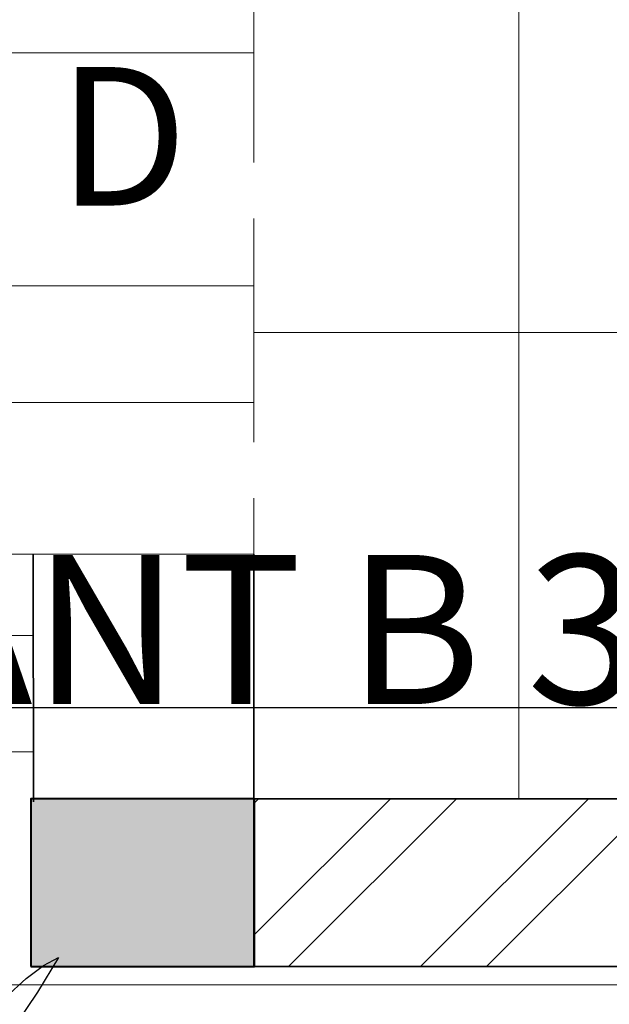
# Model space of a CAD drawing. Units: inches. Extents: x 351 to 1738, y -265 to 286.
# Tile 18 of 38: x 1236 to 1268, y -175 to -122. Entities that reach past the tile are written whole.
import ezdxf

# ---------------------------------------------------------------- set-up
doc = ezdxf.new("R2010")
doc.units = ezdxf.units.IN
doc.header["$MEASUREMENT"] = 0
doc.linetypes.add('ACAD_ISO02W100', pattern=[15, 12, -3])
for name, color, linetype, lineweight in [('A-ANNO-DIMS', 2, 'Continuous', 18), ('A-ANNO-SYMB', 7, 'Continuous', 18), ('A-COLS', 7, 'Continuous', 40), ('A-COLS-PATT', 6, 'Continuous', 13), ('A-DOOR', 3, 'Continuous', 18), ('A-DOOR-OVHD', 3, 'ACAD_ISO02W100', 13), ('A-FLOR-PATT', 9, 'Continuous', 9), ('A-WALL', 7, 'Continuous', 35), ('A-WALL-PATT', 152, 'Continuous', 13)]:
    doc.layers.add(name, color=color, linetype=linetype, lineweight=lineweight)
doc.layers.add('CAY', color=94, linetype='Continuous')
doc.layers.add('DIENHOA', color=3, linetype='Continuous')
doc.styles.add('Annotative', font='arial.ttf')
doc.styles.get("Standard").update_dxf_attribs({"font": 'arial.ttf'})
doc.dimstyles.get("Standard").update_dxf_attribs({"dimtxt": 8, "dimasz": 5, "dimexe": 0.18, "dimexo": 0.0625, "dimgap": 0.09, "dimtad": 1, "dimtoh": 1, "dimzin": 0, "dimdsep": 46, "dimlunit": 4, "dimtxsty": 'Standard', "dimcen": 0, "dimclre": 256, "dimadec": 0, "dimazin": 0, "dimtfac": 1, "dimtofl": 0, "dimtmove": 0, "dimatfit": 3, "dimfxl": 1, "dimtolj": 1, "dimtzin": 0, "dimlwe": -1, "dimarcsym": 0})

# ---------------------------------------------------------------- blocks, each defined once
blk = doc.blocks.new('Cay03_mb')
at = {"layer": 'DIENHOA'}
for points in [[(384.3, 437.5), (342.2, 367.8), (298.1, 301.7), (252.6, 239.4), (206.1, 181.1), (159.4, 127.2), (113, 78), (67.6, 33.6), (23.7, -5.4)], [(23.7, -5.4), (79.9, 91.7), (134.1, 176.2), (185.8, 248.4), (234.3, 308.7), (279, 357.3), (319.3, 394.8), (354.6, 421.4), (384.3, 437.5)]]:
    blk.add_lwpolyline(points, dxfattribs=at)
blk = doc.blocks.new('COL-9x12')
blk.add_lwpolyline([(0, 12), (0, 0), (9, 0), (9, 12)], close=True)
blk = doc.blocks.new('*D38')
at = {"layer": 'A-ANNO-DIMS', "color": 0, "lineweight": -2, "transparency": 16777216}
for p, q in [((1215.465, -164.135), (1215.465, -159.135)), ((1215.465, -159.135), (1313.607, -159.135)), ((1215.465, -195.235), (1215.465, -169.135))]:
    blk.add_line(p, q, dxfattribs=at)
at = {"layer": 'A-ANNO-DIMS', "transparency": 16777216}
for p, q in [((1210.112, -164.135), (1215.645, -164.135)), ((1210.112, -200.235), (1215.645, -200.235))]:
    blk.add_line(p, q, dxfattribs=at)
at = {"layer": 'A-ANNO-DIMS', "color": 0, "transparency": 16777216}
for points in [[(1214.631, -169.135), (1216.298, -169.135), (1215.465, -164.135)], [(1214.631, -195.235), (1216.298, -195.235), (1215.465, -200.235)]]:
    blk.add_solid(points, dxfattribs=at)
at = {"layer": 'Defpoints', "color": 0, "transparency": 16777216}
for p in [(1210.05, -164.135), (1215.465, -164.135), (1210.05, -200.235)]:
    blk.add_point(p, dxfattribs=at)
at = {"layer": 'A-ANNO-DIMS', "color": 0, "transparency": 16777216, "insert": (1264.581, -154.958), "char_height": 8, "attachment_point": 5}
blk.add_mtext('\\A1;PLANT B 3\'-0" TYP.', dxfattribs=at)
blk = doc.blocks.new('*D65')
at = {"layer": 'A-ANNO-DIMS', "transparency": 16777216}
for p, q in [((1248.45, -102.915), (1218.882, -102.915)), ((1248.45, -150.915), (1218.882, -150.915))]:
    blk.add_line(p, q, dxfattribs=at)
at = {"layer": 'A-ANNO-DIMS', "color": 0, "lineweight": -2, "transparency": 16777216}
blk.add_line((1219.062, -145.915), (1219.062, -107.915), dxfattribs=at)
at = {"layer": 'A-ANNO-DIMS', "color": 0, "transparency": 16777216}
for points in [[(1218.229, -107.915), (1219.896, -107.915), (1219.062, -102.915)], [(1218.229, -145.915), (1219.896, -145.915), (1219.062, -150.915)]]:
    blk.add_solid(points, dxfattribs=at)
at = {"layer": 'Defpoints', "color": 0, "transparency": 16777216}
for p in [(1219.062, -102.915), (1248.512, -102.915), (1248.512, -150.915)]:
    blk.add_point(p, dxfattribs=at)
at = {"layer": 'A-ANNO-DIMS', "color": 0, "transparency": 16777216, "insert": (1214.888, -126.915), "char_height": 8, "attachment_point": 5, "rotation": 90}
blk.add_mtext('\\A1;4\'-0"', dxfattribs=at)

msp = doc.modelspace()

# ---------------------------------------------------------------- hatches: boundary and pattern name
at = {"layer": 'A-COLS-PATT'}
h = msp.add_hatch(color=256, dxfattribs=at)
h.dxf.hatch_style = 1
h.paths.add_polyline_path([(1112.704, 237.963), (1103.704, 237.963), (1103.704, 228.963), (1112.704, 228.963)])
h.paths.add_polyline_path([(1115.704, 237.963), (1112.704, 237.963), (1112.704, 228.963), (1115.704, 228.963)])
h.paths.add_polyline_path([(1043.704, 255.963), (1034.704, 255.963), (1034.704, 243.963), (1043.704, 243.963)])
h.paths.add_polyline_path([(1043.704, 210.963), (1034.704, 210.963), (1034.704, 198.963), (1043.704, 198.963)])
h.paths.add_polyline_path([(1043.704, -45.037), (1034.704, -45.037), (1034.704, -57.037), (1043.704, -57.037)])
h.paths.add_polyline_path([(1112.704, -45.037), (1103.704, -45.037), (1103.704, -57.037), (1112.704, -57.037)])
h.paths.add_polyline_path([(1112.704, -161.037), (1103.704, -161.037), (1103.704, -164.037), (1103.704, -173.037), (1112.704, -173.037)])
h.paths.add_polyline_path([(1043.704, -161.037), (1034.704, -161.037), (1034.704, -173.037), (1043.704, -173.037)])
h.paths.add_polyline_path([(1248.549, -164.037), (1236.549, -164.037), (1236.549, -173.037), (1248.549, -173.037)])
h.paths.add_polyline_path([(1248.549, -50), (1236.549, -50), (1236.549, -59), (1248.549, -59)])
h.paths.add_polyline_path([(1248.704, 73.463), (1244.704, 73.463), (1244.704, 64.463), (1248.704, 64.463)])
h.paths.add_polyline_path([(1244.704, 73.463), (1236.704, 73.463), (1236.704, 64.463), (1244.704, 64.463)])
h.paths.add_polyline_path([(1248.704, 237.963), (1236.704, 237.963), (1236.704, 228.963), (1248.704, 228.963)])
h.paths.add_polyline_path([(1392.204, 237.963), (1380.204, 237.963), (1380.204, 228.963), (1392.204, 228.963)])
h.paths.add_polyline_path([(1536.064, 237.963), (1524.064, 237.963), (1524.064, 228.963), (1536.064, 228.963)])
h.paths.add_polyline_path([(1536.064, 73.463), (1524.064, 73.463), (1524.064, 64.463), (1536.064, 64.463)])
h.paths.add_polyline_path([(1384.204, 73.463), (1380.204, 73.463), (1380.204, 64.463), (1384.204, 64.463)])
h.paths.add_polyline_path([(1392.064, 73.463), (1384.204, 73.463), (1384.204, 64.463), (1392.064, 64.463)])
h.paths.add_polyline_path([(1536.064, -53.037), (1524.064, -53.037), (1524.064, -57.037), (1536.064, -57.037)])
h.paths.add_polyline_path([(1536.064, -48.037), (1524.064, -48.037), (1524.064, -53.037), (1536.064, -53.037)])
h.paths.add_polyline_path([(1392.064, -48.037), (1380.064, -48.037), (1380.064, -56.5), (1380.065, -57.037), (1392.064, -57.037)])
h.paths.add_polyline_path([(1536.064, -164.037), (1524.064, -164.037), (1524.064, -173.037), (1536.064, -173.037)])
at = {"layer": 'A-FLOR-PATT', "transparency": 33554559}
h = msp.add_hatch(dxfattribs=at)
h.set_pattern_fill('ANSI37', color=256, scale=200, angle=135)
h.set_pattern_definition([(180, (1112.704, -164.037), (-2e-15, -25), []), (270, (1112.704, -164.037), (25, -5e-15), [])])
h.paths.add_polyline_path([(1380.064, 73.463), (1380.132, 148.463), (1338.064, 148.463), (1290.704, 148.463), (1290.704, 88.463), (1248.704, 88.463), (1248.704, -2.009), (1244.704, -2.009), (1244.704, 142.457), (1160.704, 142.457), (1160.704, 158.963), (1160.704, 170.137), (1160.704, 206.137), (1160.704, 228.963), (1112.704, 228.963), (1112.704, 209.963), (1112.704, 168.963), (1124.704, 168.963), (1124.704, 162.963), (1112.704, 162.963), (1112.704, 64.463), (1112.704, 60.463), (1112.704, 0.463), (1112.704, -48.026), (1146.804, -47.981), (1146.804, -35.691), (1207.804, -35.691), (1207.804, -47.902), (1236.542, -47.864), (1236.544, -50.009), (1248.5, -50.009), (1248.506, -102.915), (1248.512, -150.915), (1248.514, -164.037), (1248.549, -164.037), (1273.017, -164.037), (1273.017, -128.799), (1355.24, -128.799), (1355.24, -164.037), (1384.204, -164.037), (1384.204, -57.037), (1380.064, -57.037), (1380.064, -48.037), (1392.064, -48.037), (1392.064, -53.037), (1406.549, -53.037), (1406.549, -57.037), (1401.204, -57.037), (1401.204, -147.037), (1468.204, -147.037), (1468.204, -138.5), (1472.204, -138.5), (1472.204, -102.5), (1468.204, -102.5), (1468.204, -57.037), (1442.549, -57.037), (1442.549, -53.037), (1463.049, -53.037), (1463.049, -40.747), (1524.049, -40.747), (1524.049, -48.037), (1536.064, -48.037), (1536.064, -53.037), (1557.704, -53.037), (1557.704, 204.963), (1384.204, 204.963), (1384.204, 73.463), (1392.064, 73.463), (1392.064, 64.463), (1384.204, 64.463), (1384.204, -3.5), (1380.204, -3.537), (1380.204, 64.463), (1380.064, 64.463)])
h.paths.add_polyline_path([(1510.714, 86.458, -0.103984), (1511.661, 85.595, 0.470438), (1510.158, 87.614, 0.0961)], flags=16)
h.paths.add_polyline_path([(1510.443, 100.266, 0.009798), (1504.693, 100.48, 0.02879), (1504.6, 99.767, -0.165331), (1505.519, 96.135, -0.143601)], flags=16)
h.paths.add_polyline_path([(1487.201, 85.595, -0.103984), (1488.148, 86.458, 0.0961), (1488.704, 87.614, 0.470438)], flags=0)
h.paths.add_polyline_path([(1495.052, 100.43), (1494.178, 100.43, -0.026463), (1494.262, 99.774, -0.144219)], flags=16)
h.paths.add_polyline_path([(1444.485, 86.458, -0.103984), (1445.433, 85.595, 0.470438), (1443.93, 87.614, 0.0961)], flags=16)
h.paths.add_polyline_path([(1420.972, 85.595, -0.103984), (1421.92, 86.458, 0.0961), (1422.475, 87.614, 0.470438)], flags=16)
h.paths.add_polyline_path([(1428.632, 100.335, 0.001054), (1427.971, 100.309, -0.021524), (1428.033, 99.774, -0.114301)], flags=16)
h.paths.add_polyline_path([(1419.906, 143.708, 0.024979), (1420.222, 157.526), (1421.573, 159.101), (1421.573, 175.369), (1391.393, 175.369), (1391.393, 200.519), (1542.294, 200.519), (1542.294, 175.369), (1512.028, 175.369, 0.019865), (1511.521, 153.838, 0.025134), (1512.758, 118.323, 0.020553), (1512.942, 115.253), (1419.834, 115.253, -0.000414), (1419.843, 124.798), (1413.059, 124.798), (1413.059, 84.437, -0.061853), (1415.831, 80.45, -0.093077), (1420.972, 85.595, -0.267537), (1422.371, 84.732, 0.08511), (1424.052, 84.616, -0.885393), (1424.033, 84.851, -1.125815), (1424.073, 84.366, -0.087987), (1422.371, 84.732, -0.267537), (1422.326, 83.089, -0.370542), (1420.972, 85.595, 0.093077), (1415.831, 80.45, -0.087414), (1417.914, 73.937), (1418.941, 73.937, 0.02725), (1418.913, 76.906, -0.115703), (1421.051, 73.937), (1445.354, 73.937, -0.115703), (1447.492, 76.906, 0.02725), (1447.464, 73.937), (1448.491, 73.937, -0.087414), (1450.574, 80.45, 0.093077), (1445.433, 85.595, -0.370542), (1444.079, 83.089, -0.267537), (1444.034, 84.732, -0.087987), (1442.332, 84.366, -1.125815), (1442.372, 84.851, -2.032736), (1442.364, 84.368, 0.086378), (1444.034, 84.732, -0.267537), (1445.433, 85.595, -0.093077), (1450.574, 80.45, -0.257732), (1466.483, 90.927, -0.47867), (1468.832, 91.907, -0.47867), (1471.18, 90.927, -0.26264), (1483.053, 81.78, -0.071866), (1487.201, 85.595, -0.267537), (1488.6, 84.732, 0.08511), (1490.28, 84.616, -0.885393), (1490.262, 84.851, -1.125815), (1490.301, 84.366, -0.087987), (1488.6, 84.732, -0.267537), (1488.554, 83.089, -0.370542), (1487.201, 85.595, 0.071866), (1483.053, 81.78, -0.132065), (1484.143, 73.937), (1485.169, 73.937, 0.02725), (1485.142, 76.906, -0.115703), (1487.28, 73.937), (1511.582, 73.937, -0.115703), (1513.72, 76.906, 0.02725), (1513.693, 73.937), (1514.719, 73.937, -0.087414), (1516.802, 80.45, 0.093077), (1511.661, 85.595, -0.370542), (1510.308, 83.089, -0.267537), (1510.262, 84.732, -0.087987), (1508.561, 84.366, -1.125815), (1508.601, 84.851, -2.032736), (1508.592, 84.368, 0.086378), (1510.262, 84.732, -0.267537), (1511.661, 85.595, -0.093077), (1516.802, 80.45, -0.061853), (1519.575, 84.437), (1519.575, 73.937), (1413.059, 73.937), (1413.059, 124.798), (1419.843, 124.798, -0.000821)], flags=16)
h.paths.add_polyline_path([(1220.149, 54.133, -0.103984), (1220.869, 53.476, 0.470438), (1219.727, 55.011, 0.0961)], flags=16)
h.paths.add_polyline_path([(1219.944, 64.626, 0.009798), (1215.574, 64.789, 0.02879), (1215.503, 64.247, -0.165331), (1216.201, 61.487, -0.143601)], flags=16)
h.paths.add_polyline_path([(1209.779, 64.449, 0.097446), (1209.339, 64.751), (1208.247, 64.751, 0.12739), (1207.7, 64.326, 0.171586), (1206.95, 61.475, -0.158854), (1207.636, 59.45, 0.015898), (1207.795, 59.218, 0.061546), (1208.598, 59.616, 0.175416), (1208.638, 60.099, -0.284779), (1209.348, 62.472, 0.326216)], flags=16)
h.paths.add_polyline_path([(1169.818, 54.133, -0.103984), (1170.538, 53.476, 0.470438), (1169.396, 55.011, 0.0961)], flags=16)
h.paths.add_polyline_path([(1159.017, 62.472, 0.284764), (1158.307, 60.099, -0.175433), (1158.267, 59.616, 0.39293), (1159.448, 64.449, -0.32623)], flags=16)
h.paths.add_polyline_path([(1156.342, 58.239, -0.178321), (1154.011, 55.31, -0.174736), (1154.722, 55.233, -0.200802), (1156.27, 56.086, 0.12699), (1157.283, 58.991, -0.091205)], flags=16)
h.paths.add_polyline_path([(1156.624, 61.413, 0.157275), (1157.316, 64.247, 0.169622)], flags=16)
h.paths.add_polyline_path([(1152.67, 54.133, -0.0961), (1151.95, 53.476, 0.064076), (1154.465, 54.384, 0.199016)], flags=16)
h.paths.add_polyline_path([(1202.281, 53.476, -0.103984), (1203, 54.133, 0.0961), (1203.423, 55.011, 0.470438)], flags=0)
h.paths.add_polyline_path([(1151.139, 97.64, 0.024979), (1151.379, 108.141), (1152.406, 109.338), (1152.406, 121.701), (1129.47, 121.701), (1129.47, 140.814), (1244.149, 140.814), (1244.149, 121.701), (1221.148, 121.701, 0.019865), (1220.763, 105.338, 0.025134), (1221.703, 78.349, 0.020553), (1221.843, 76.016), (1151.078, 76.016, -0.128743), (1148.786, 65.037, 0.539352), (1150.327, 64.171, -0.027594), (1163.481, 64.751, 0.097695), (1163.04, 64.449, 0.326216), (1163.471, 62.472, -0.284777), (1164.181, 60.099, -0.194757), (1165.846, 61.443, -0.155402), (1165.172, 64.247, -0.166022), (1165.869, 61.475, -0.177014), (1167.852, 62.77, -0.448203), (1169.974, 60.807, -0.393499), (1167.679, 57.86, -0.895548), (1168.438, 54.524, -0.355767), (1166.218, 56.086, -0.066024), (1165.505, 57.539), (1165.251, 56.243, -0.371732), (1164.02, 59.758, -0.373614), (1163.04, 64.449, -0.097695), (1163.481, 64.751, 0.021354), (1153.294, 64.429, -0.134183), (1156.695, 61.368, 0.186873), (1154.636, 62.77, 0.448203), (1152.514, 60.807, 0.403726), (1154.905, 57.846, 0.711219), (1153.334, 55, 0.53154), (1151.95, 53.476, -0.267537), (1153.013, 52.821, 0.08511), (1154.29, 52.732, -0.885393), (1154.276, 52.911, -1.125815), (1154.306, 52.543, -0.087987), (1153.013, 52.821, -0.267537), (1152.978, 51.572, -0.370542), (1151.95, 53.476, 0.093077), (1148.043, 49.566, -0.087414), (1149.626, 44.617), (1150.406, 44.617, 0.02725), (1150.385, 46.873, -0.115703), (1152.01, 44.617), (1170.478, 44.617, -0.115703), (1172.103, 46.873, 0.02725), (1172.082, 44.617), (1172.862, 44.617, -0.087414), (1174.445, 49.566, 0.093077), (1170.538, 53.476, -0.370542), (1169.51, 51.572, -0.267537), (1169.475, 52.821, -0.087987), (1168.182, 52.543, -1.125815), (1168.212, 52.911, -2.032736), (1168.206, 52.544, 0.086378), (1169.475, 52.821, -0.267537), (1170.538, 53.476, -0.093077), (1174.445, 49.566, -0.257732), (1186.536, 57.528, -0.47867), (1188.321, 58.273, -0.47867), (1190.106, 57.528, -0.26264), (1199.128, 50.577, -0.071866), (1202.281, 53.476, -0.267537), (1203.344, 52.821, 0.08511), (1204.621, 52.732, -0.885393), (1204.607, 52.911, -1.125815), (1204.637, 52.543, -0.087987), (1203.344, 52.821, -0.267537), (1203.309, 51.572, -0.370542), (1202.281, 53.476, 0.071866), (1199.128, 50.577, -0.132065), (1199.957, 44.617), (1200.737, 44.617, 0.02725), (1200.716, 46.873, -0.115703), (1202.341, 44.617), (1220.809, 44.617, -0.115703), (1222.434, 46.873, 0.02725), (1222.413, 44.617), (1223.193, 44.617, -0.087414), (1224.776, 49.566, 0.093077), (1220.869, 53.476, -0.370542), (1219.841, 51.572, -0.267537), (1219.806, 52.821, -0.087987), (1218.513, 52.543, -1.125815), (1218.543, 52.911, -2.032736), (1218.537, 52.544, 0.086378), (1219.806, 52.821, -0.267537), (1220.869, 53.476, -0.093077), (1224.776, 49.566, -0.061853), (1226.883, 52.597), (1226.883, 44.617), (1145.936, 44.617), (1145.936, 83.269), (1151.091, 83.269, -0.000821)], flags=16)
h.paths.add_polyline_path([(1218.01, 57.86, -0.895548), (1218.769, 54.524, -0.355767), (1216.549, 56.086, -0.066024), (1215.836, 57.539), (1215.582, 56.243, -0.371732), (1214.351, 59.758, -0.373614), (1213.371, 64.449, 0.326216), (1213.802, 62.472, -0.284777), (1214.512, 60.099, -0.194757), (1216.177, 61.443, -0.179991), (1218.183, 62.77, -0.448203), (1220.305, 60.807, -0.393499)], flags=16)
h.paths.add_polyline_path([(1424.735, 91.363, -0.393499), (1421.715, 95.241, -0.448203), (1424.507, 97.824, -0.179991), (1427.147, 96.077, -0.194757), (1429.338, 94.309, -0.284777), (1430.272, 97.432, 0.326216), (1430.839, 100.034, -0.373614), (1429.55, 93.861, -0.371732), (1427.929, 89.235), (1427.596, 90.941, -0.066024), (1426.657, 89.029, -0.355767), (1423.736, 86.973, -0.895548)], flags=16)
h.paths.add_polyline_path([(1238.033, 131.257, -1), (1227.329, 131.257, -1)], flags=0)
h.paths.add_polyline_path([(1235.357, 131.257, -1), (1230.005, 131.257, -1)], flags=0)
h.paths.add_polyline_path([(1214.039, 54.243, 0.154382), (1214.38, 53.992, 0.358955), (1213.613, 54.016, 0.603948), (1214.379, 53.657, 0.371319), (1213.968, 52.872, 0.187994), (1214.312, 52.809, -0.592455), (1213.953, 52.967, -0.294279), (1214.083, 53.691, -1.300187), (1213.881, 54.134, -0.283762), (1214.469, 53.896, 1.15094)], flags=16)
h.paths.add_polyline_path([(1212.091, 56.286, -0.408434), (1211.337, 56.445, -0.036259), (1211.098, 56.848, -0.236098), (1211.59, 56.63, 0.035345), (1211.835, 56.543, -0.475241), (1212.091, 56.286, -0.475241), (1212.438, 56.182, 0.035345), (1212.631, 56.007, -0.236098), (1213.056, 55.676, -0.036259), (1212.588, 55.697, -0.408434)], flags=16)
h.paths.add_polyline_path([(1211.469, 50.297, 0.296043), (1210.47, 50.527, 0.310883), (1211.931, 50.148, 0.021255)], flags=16)
h.paths.add_polyline_path([(1213.739, 51.818, -0.036259), (1213.271, 51.838, -0.408434), (1212.774, 52.427, -0.094786), (1212.293, 50.703, 1.150474), (1212.911, 50.232, 0.166288), (1213.265, 50.68, -0.025254), (1212.603, 50.13, 1.087932), (1212.471, 49.407, 0.166288), (1213.02, 49.251, -0.016128), (1212.567, 49.563, -0.286859), (1212.217, 49.638, 0.022156), (1212.046, 50.055, -0.64613), (1212.185, 50.498, 0.088412), (1212.732, 52.077, -1.186037), (1213.121, 52.323, 0.035345), (1213.314, 52.148, -0.236098)], flags=16)
h.paths.add_polyline_path([(1212.094, 50.342, -0.048524), (1211.54, 49.605, -1.103834), (1211.397, 48.738, -0.785515), (1211.683, 48.254, -0.392043), (1210.948, 48.525, -0.392819), (1210.561, 47.995, -0.592455), (1210.201, 48.153, -0.294279), (1210.331, 48.877, -0.704172), (1210.316, 49.592, -0.679344), (1210.729, 50.112, 0.563676)], flags=16)
h.paths.add_polyline_path([(1211.274, 49.829, -0.139826), (1210.745, 49.859, -0.217879), (1210.948, 49.509, -0.498572)], flags=0)
h.paths.add_polyline_path([(1433.426, 81.49, -0.181571), (1434.245, 81.788, -0.008067), (1433.726, 82.205, 0.045578), (1432.755, 81.242, 0.179011)], flags=16)
h.paths.add_polyline_path([(1434.146, 81.009, -0.132442), (1433.645, 80.771, 0.259089), (1433.234, 80.471, -0.180211), (1433.392, 80.805, -0.16994), (1432.758, 81.109, 0.032652), (1433.273, 80.474, -0.493363), (1434.046, 80.146, -0.390497)], flags=16)
h.paths.add_polyline_path([(1434.83, 80.047, -0.947538), (1435.294, 79.576, -0.299128), (1434.625, 79.404, -0.270439), (1435.01, 78.591, -0.592455), (1434.537, 78.382, -0.392819), (1434.027, 79.08, -0.392043), (1433.06, 78.723, -0.352042), (1433.003, 79.197, -0.197216), (1433.75, 79.734, -0.71364), (1434.447, 79.939, -0.21479), (1434.819, 80.475, 0.408833), (1435.075, 80.803, -0.226152)], flags=16)
h.paths.add_polyline_path([(1432.67, 81.217, -0.454218), (1431.897, 79.923, -0.414411), (1431.301, 80.035, 0.016129), (1431.897, 80.445, 0.27957), (1432.073, 80.871, -0.289504), (1431.103, 81.321, -0.414411), (1430.978, 81.915, 0.01613), (1431.586, 81.521, 0.341293), (1432.125, 81.583, -0.813186)], flags=16)
h.paths.add_polyline_path([(1429.893, 86.381, -0.947538), (1430.358, 85.91, -0.173106), (1429.984, 85.712, -0.038817), (1431.625, 84.214, -0.0879), (1432.097, 88.549, -0.049768), (1431.254, 88.49, -0.236098), (1431.814, 88.925, 0.035345), (1432.067, 89.155, -0.475241), (1432.524, 89.291, -0.475241), (1432.86, 89.63, 0.035345), (1433.182, 89.744, -0.236098), (1433.83, 90.032, -0.036259), (1433.516, 89.502, -0.408434), (1432.524, 89.291, -0.312424), (1432.106, 88.58, 0.088559), (1431.625, 84.214, -0.408434), (1430.971, 83.439, -0.036259), (1430.355, 83.412, -0.236098), (1430.914, 83.847, 0.035345), (1431.168, 84.078, -0.475241), (1431.625, 84.214, 0.038817), (1429.984, 85.712, -0.321732), (1429.333, 86.048, -0.32743), (1429.883, 86.809, 0.408833), (1430.138, 87.138, -0.226152)], flags=16)
h.paths.add_polyline_path([(1211.206, 58.616, -0.999784), (1211.336, 59.323, -0.614994)], flags=16)
h.paths.add_polyline_path([(1210.288, 49.429, 0.154382), (1210.629, 49.178, 0.358955), (1209.861, 49.202, 0.603948), (1210.627, 48.843, -0.534825), (1210.806, 49.295, 0.748346)], flags=16)
h.paths.add_polyline_path([(1209.589, 51.828, -0.008791), (1209.775, 51.753, 0.112231), (1209.466, 52.019, 1.418851), (1209.014, 51.708, -0.458726), (1208.651, 51.073, -0.592455), (1208.291, 51.232, -0.294279), (1208.421, 51.955, -1.300187), (1208.219, 52.398, -0.226005), (1208.719, 52.257, -0.475519), (1209.158, 52.369, -1.455499), (1209.603, 52.664, 0.421305), (1209.191, 52.262, -0.591212), (1208.979, 51.796, 0.497399), (1209.773, 51.333, 0.649312)], flags=16)
h.paths.add_polyline_path([(1208.029, 52.041, 0.544667), (1208.832, 52.045, 0.220132)], flags=0)
h.paths.add_polyline_path([(1210.438, 51.425, -0.2042), (1210.277, 52.018, 0.270826), (1209.915, 52.897, 0.324115)], flags=0)
h.paths.add_polyline_path([(1209.668, 52.407, -0.60139), (1208.99, 52.221, -0.394916), (1208.248, 52.83, -0.836792), (1208.651, 53.017, -0.338488), (1209.039, 52.571, 0.194138), (1209.191, 52.262, 0.413995), (1209.712, 52.475, 0.51771), (1210.503, 51.416, 0.401922), (1209.493, 50.93, 0.206396), (1209.516, 50.165, -0.319463), (1210.417, 51.418, -0.466635)], flags=16)
h.paths.add_polyline_path([(1206.601, 56.086, -0.355767), (1204.381, 54.524, -0.921198), (1205.236, 57.846, 0.206569), (1207.614, 58.991, -0.12699)], flags=16)
h.paths.add_polyline_path([(1435.487, 82.816, 0.527765), (1436.615, 83.361, 0.50854), (1437.05, 82.433, 0.592455), (1437.524, 82.641, 0.331245), (1436.963, 83.548, 0.387863), (1437.808, 83.626, 0.592954), (1437.618, 84.176, 0.226016), (1436.961, 83.99, 0.318205), (1437.588, 84.854, 0.689374), (1437.05, 84.991, 0.335765), (1436.539, 84.41, -0.156993), (1436.404, 84.065, -0.434611), (1436.961, 83.99, -0.21479), (1437.333, 84.526, 0.408833), (1437.588, 84.854, -0.226152), (1437.343, 84.097, -0.947538), (1437.808, 83.626, -0.299128), (1437.139, 83.455, -0.270439), (1437.524, 82.641, -0.592455), (1437.05, 82.433, -0.392819), (1436.541, 83.13, -0.43966), (1435.475, 82.794, -0.174614), (1435.942, 82.244, -0.206396), (1435.912, 81.237, -0.270826), (1435.125, 82.208, 0.207976), (1434.686, 82.904, -0.196495)], flags=16)
h.paths.add_polyline_path([(1435.386, 84.832, 0.270811), (1434.91, 83.676, -0.204217), (1434.699, 82.895, 0.324115)], flags=0)
h.paths.add_polyline_path([(1435.68, 84.18, -0.217656), (1435.554, 83.304, -0.176705), (1436.236, 83.778, -0.373036)], flags=0)
h.paths.add_polyline_path([(1435.566, 100.034, 0.326216), (1436.133, 97.432, -0.284777), (1437.067, 94.309, -0.194757), (1439.258, 96.077, -0.155402), (1438.371, 99.767, -0.166022), (1439.289, 96.12, -0.177014), (1441.897, 97.824, -0.448203), (1444.69, 95.241, -0.393499), (1441.67, 91.363, -0.895548), (1442.669, 86.973, -0.355767), (1439.748, 89.029, -0.066024), (1438.809, 90.941), (1438.476, 89.235, -0.371732), (1436.855, 93.861, -0.373614)], flags=16)
h.paths.add_polyline_path([(1191.252, 49.507, -0.274022), (1190.658, 48.409, 0.267537), (1191.311, 47.344, 0.370542)], flags=0)
h.paths.add_polyline_path([(1190.301, 49.717, 0.199016), (1188.619, 49.04, 0.064076), (1191.252, 49.507, -0.0961)], flags=0)
h.paths.add_polyline_path([(1189.518, 47.857, 1.125815), (1189.676, 47.523, 2.044605)], flags=0)
h.paths.add_polyline_path([(1464.974, 80.372, 0.274022), (1465.756, 78.927, -0.083013)], flags=0)
h.paths.add_polyline_path([(1464.974, 80.372, 0.370542), (1464.897, 77.525, 0.576324)], flags=0)
h.paths.add_polyline_path([(1464.974, 80.372, -0.470438), (1467.284, 81.372, -0.0961), (1466.226, 80.648, -0.199016), (1468.439, 79.757, -0.064076)], flags=0)
h.paths.add_polyline_path([(1189.511, 56.43, -0.259467), (1188.321, 56.391, -0.259467), (1187.13, 56.43, 0.08511), (1188.193, 55.716, -0.885393), (1188.27, 55.878, -1.196013), (1188.355, 55.442, 0.101459)], flags=0)
h.paths.add_polyline_path([(1188.321, 57.596, 0.078072), (1187.678, 57.24, 0.01555), (1188.321, 57.136, 0.01555), (1188.964, 57.24, 0.078072)], flags=0)
h.paths.add_polyline_path([(1190.164, 55.365, -0.576324), (1190.106, 57.528, -0.198294), (1188.321, 58.319, -0.198294), (1186.536, 57.528, -0.576324), (1186.477, 55.365, -0.370542), (1186.536, 57.528, 0.198294), (1188.321, 58.319, 0.198294), (1190.106, 57.528, -0.370542)], flags=0)
h.paths.add_polyline_path([(1188.372, 55.878, 1.125814), (1188.529, 55.544, 2.044605)], flags=0)
h.paths.add_polyline_path([(1186.341, 49.717, -0.0961), (1185.389, 49.507, 0.064076), (1188.022, 49.04, 0.199016)], flags=0)
h.paths.add_polyline_path([(1185.389, 49.507, -0.267537), (1185.984, 48.409, 0.08511), (1187.046, 47.695, -0.885393), (1187.123, 47.857, -1.125815), (1186.966, 47.523, -0.087987), (1185.984, 48.409, -0.267537), (1185.331, 47.344, -0.370542)], flags=0)
h.paths.add_polyline_path([(1399.441, 187.944, -1), (1413.525, 187.944, -1)], flags=0)
h.paths.add_polyline_path([(1402.962, 187.944, -1), (1410.004, 187.944, -1)], flags=0)
h.paths.add_polyline_path([(1357.663, -72.245), (1377.272, -72.245), (1377.272, -91.854), (1357.663, -91.854)], flags=16)
h.paths.add_polyline_path([(1467.256, 78.201, -1.125815), (1467.049, 77.761, -2.044605)], flags=0)
h.paths.add_polyline_path([(1468.822, 88.714, 0.941125), (1469.106, 88.316, 1.137152), (1468.765, 88.755, 0.890986), (1468.99, 88.245, 0.094828), (1470.398, 89.481, -0.267537), (1471.18, 90.927, -0.028123), (1469.678, 90.547, -0.028774), (1469.948, 90.311, -0.020327), (1468.832, 90.41, -0.020327), (1467.716, 90.311, -0.028774), (1467.986, 90.547, -0.028123), (1466.483, 90.927, -0.267537), (1467.265, 89.481, 0.08511), (1468.663, 88.542, -1.202316)], flags=0)
h.paths.add_polyline_path([(1178.25, 124.523, -0.119929), (1165.65, 124.145, -0.107349), (1159.133, 124.446, -0.102891), (1159.132, 130.465, -0.074897), (1158.993, 137.956, 0.002027), (1167.844, 137.479, -0.07553), (1180.337, 137.666, -0.075861), (1186.502, 137.688, -0.14099), (1186.272, 130.046, -0.095481), (1186.729, 124.748, -0.10603)], flags=0)
h.paths.add_polyline_path([(1469.225, 79.757, -0.199016), (1471.437, 80.648, -0.0961), (1470.379, 81.372, -0.470438), (1472.689, 80.372, -0.370542), (1472.766, 77.525, -0.267537), (1471.907, 78.927, -0.087986), (1470.615, 77.761, -1.125849), (1470.408, 78.201, -2.032736), (1470.642, 77.778, 0.086378), (1471.907, 78.927, -0.267537), (1472.689, 80.372, -0.064076)], flags=0)
h.paths.add_polyline_path([(1430.423, 186.902, -0.074897), (1430.24, 196.758, 0.002027), (1441.887, 196.131, -0.07553), (1458.326, 196.377, -0.075861), (1466.438, 196.406, -0.14099), (1466.136, 186.35, -0.095481), (1466.737, 179.378, -0.10603), (1455.58, 179.082, -0.119929), (1439, 178.585, -0.107349), (1430.425, 178.981, -0.102891)], flags=0)
h.paths.add_polyline_path([(1162.258, 49.939, 0.335765), (1161.87, 49.497, -0.156994), (1161.767, 49.235, -0.434611), (1162.19, 49.178, -0.21479), (1162.473, 49.585, 1.529195)], flags=16)
h.paths.add_polyline_path([(1161.683, 49.021, 0.581518), (1161.268, 49.583, 0.592761)], flags=16)
h.paths.add_polyline_path([(1162.602, 48.058, 0.371319), (1162.192, 48.843, 0.434533), (1162.88, 48.962, 0.185081), (1162.197, 48.926, 1.121837)], flags=16)
h.paths.add_polyline_path([(1161.443, 48.941, -1.307104), (1161.495, 48.571, -0.217752), (1161.136, 48.254, 0.697303), (1161.871, 49.048, 0.121514)], flags=16)
h.paths.add_polyline_path([(1162.531, 49.429, -0.207084), (1162.05, 49.146, -0.99203)], flags=16)
h.paths.add_polyline_path([(1161.304, 49.578, -0.719667), (1161.513, 50.079, -0.130428), (1160.836, 50.168, 0.039593)], flags=0)
h.paths.add_polyline_path([(1162.036, 50.584, -0.008067), (1161.642, 50.9, 0.029367), (1161.35, 50.297, -0.205788)], flags=16)
h.paths.add_polyline_path([(1162.882, 51.392, -0.124733), (1162.763, 51.828, -0.101191), (1162.399, 51.438, -0.153425)], flags=0)
h.paths.add_polyline_path([(1164.235, 51.85, -0.309107), (1164.513, 51.136, -0.627125), (1163.781, 51.603, -0.685909), (1162.777, 51.219, -0.233285), (1163.303, 50.165, -0.270826), (1162.705, 50.903, 0.2042), (1162.381, 51.425, 0.204182), (1162.542, 52.018, -0.270841), (1162.903, 52.897, -0.127261), (1163.219, 52.529, -1.168681), (1163.781, 52.587, -0.329112), (1164.168, 53.017, -0.836792), (1164.571, 52.83, -0.193341), (1164.391, 52.338, -0.947538), (1164.744, 51.981, -0.299128)], flags=16)
h.paths.add_polyline_path([(1163.598, 51.937, -1.262956), (1163.236, 51.831, 0.012575), (1162.971, 51.721, 0.230657), (1163.151, 52.407, -0.164898), (1163.178, 52.661, -0.44932), (1163.628, 52.262, -0.721477), (1164.154, 52.088, -0.849998)], flags=0)
h.paths.add_polyline_path([(1161.613, 58.616, -0.980413), (1161.525, 59.049, -2.908935)], flags=16)
h.paths.add_polyline_path([(1160.252, 49.166, -0.414411), (1159.799, 49.251, 0.016129), (1160.252, 49.563, 0.27957), (1160.386, 49.887, -0.289504), (1159.649, 50.229, -0.414411), (1159.554, 50.68, 0.01613), (1160.015, 50.381, 0.617885), (1160.526, 50.703, -0.094786), (1160.045, 52.427, -0.140444), (1159.682, 52.042, -0.057856), (1159.3, 51.872, 0.544843), (1160.046, 52.419, -0.088122), (1160.404, 55.721, -0.049768), (1159.763, 55.676, -0.236098), (1160.188, 56.007, 0.035345), (1160.381, 56.182, -0.475241), (1160.728, 56.286, -0.475241), (1160.984, 56.543, 0.035345), (1161.229, 56.63, -0.236098), (1161.721, 56.848, -0.036259), (1161.482, 56.445, -0.408434), (1160.728, 56.286, -0.312424), (1160.411, 55.745, 0.088559), (1160.045, 52.427, 0.107081), (1160.634, 50.498, -0.494798), (1160.839, 50.149, -0.454218)], flags=16)
h.paths.add_polyline_path([(1160.666, 49.808, -2.076528), (1160.828, 50.172, 0.019586)], flags=0)
h.paths.add_polyline_path([(1158.439, 53.992, 0.154382), (1158.78, 54.243, 0.748346), (1158.262, 54.109, -0.338225), (1158.492, 53.839, -0.170816), (1159.124, 53.779, 0.495729), (1158.938, 54.134, 0.226016)], flags=16)
h.paths.add_polyline_path([(1160.045, 52.427, 0.038817), (1158.798, 53.565, -0.119818), (1158.574, 53.586, -0.309107), (1158.851, 52.872, -0.187994), (1158.506, 52.809, 0.592455), (1158.866, 52.967, 0.331245), (1158.44, 53.657, 0.201245), (1158.798, 53.565, -0.034023), (1159.901, 52.578, -0.044253), (1159.698, 52.323, -0.475241)], flags=16)
h.paths.add_polyline_path([(1336.926, -95.392), (1336.926, -117.945), (1291.82, -117.945), (1291.82, -95.392)], flags=16)
h.paths.add_polyline_path([(1357.535, -97.244), (1357.726, -96.697, 0.034844)], flags=16)
h.paths.add_polyline_path([(1376.693, -96.478), (1377.301, -96.5, 0.031497), (1375.907, -96.424), (1357.726, -96.424)], flags=16)
h.paths.add_polyline_path([(1379.403, -119.667, 0.026706), (1380.043, -119.439, -0.015299)], flags=16)
h.paths.add_polyline_path([(1357.726, -120.202), (1357.821, -120.202), (1357.821, -120.201)], flags=16)
h.paths.add_polyline_path([(1354.171, -104.592), (1354.469, -98.672, 0.011138)], flags=16)
h.paths.add_polyline_path([(1355.058, -119.136), (1354.578, -118.539, 0.143164)], flags=16)
h.paths.add_polyline_path([(1378.851, -96.821), (1378.85, -96.82), (1378.85, -96.82, -0.04968), (1380.055, -97.191), (1378.85, -96.82, 0.150054), (1375.135, -97.188), (1375.136, -119.44, -0.00997), (1374.747, -116.649), (1357.726, -116.649, 0.169385), (1357.535, -119.382), (1357.535, -119.382), (1357.535, -119.382, 0.034818), (1357.726, -119.928), (1357.726, -119.928), (1357.726, -119.929, -0.034877), (1357.535, -119.382), (1355.507, -119.382), (1355.317, -119.278), (1357.535, -119.382, -0.169394), (1357.726, -116.649, -0.039151), (1374.686, -116.113, -0.002015), (1374.625, -115.546, 0.115322), (1369.915, -115.474, 0.060921), (1369.922, -101.154, 0.115146), (1374.625, -101.079, -0.002016), (1374.686, -100.513, -0.039151), (1357.726, -99.977), (1374.747, -99.977, -0.009963), (1375.135, -97.188), (1375.135, -97.188, -0.150108)], flags=16)
h.paths.add_polyline_path([(1490.963, 91.363, -0.393499), (1487.944, 95.241, -0.448203), (1490.736, 97.824, -0.179991), (1493.376, 96.077, -0.194757), (1495.567, 94.309, -0.284777), (1496.501, 97.432, 0.326216), (1497.068, 100.034, -0.373614), (1495.778, 93.861, -0.371732), (1494.158, 89.235), (1493.824, 90.941, -0.066024), (1492.886, 89.029, -0.355767), (1489.964, 86.973, -0.895548)], flags=16)
h.paths.add_polyline_path([(1354.86, -97.658), (1355.316, -97.348, 0.101911)], flags=16)
h.paths.add_polyline_path([(1497.063, 83.327, 0.176724), (1496.37, 83.785, -0.405139), (1496.016, 83.384, 0.497399), (1497.06, 82.774, 0.649312), (1496.818, 83.426, -0.008791)], flags=16)
h.paths.add_polyline_path([(1496.339, 83.783, 0.592761), (1496.886, 84.522, 0.581518)], flags=16)
h.paths.add_polyline_path([(1495.11, 82.641, 0.592455), (1495.583, 82.433, 0.676915), (1495.805, 83.59, 0.375669)], flags=16)
h.paths.add_polyline_path([(1495.015, 84.176, -0.145057), (1495.301, 84.526, -0.408833), (1495.045, 84.854, 0.220629), (1495.381, 84.152, -0.199594), (1495.851, 83.764, -0.524017), (1494.826, 83.626, -0.592998)], flags=16)
h.paths.add_polyline_path([(1501.655, 81.915, -0.016129), (1501.048, 81.521, -0.392719), (1500.462, 81.37, -0.21067), (1500.607, 81.142, 0.306699)], flags=16)
h.paths.add_polyline_path([(1500.11, 89.291, -0.408434), (1499.118, 89.502, -0.036259), (1498.803, 90.032, -0.236098), (1499.451, 89.744, 0.035345), (1499.774, 89.63, -0.475241), (1500.11, 89.291, -0.475241), (1500.567, 89.155, 0.035345), (1500.82, 88.925, -0.236098), (1501.379, 88.49, -0.036259), (1500.763, 88.516, -0.408434)], flags=16)
h.paths.add_polyline_path([(1498.908, 82.205, -0.051322), (1500.013, 81.134, -0.587931), (1500.234, 81.676, 0.107081), (1501.009, 84.214, -0.03529)], flags=16)
h.paths.add_polyline_path([(1496.93, 83.875, -0.206396), (1497.247, 84.832, -0.270826), (1497.724, 83.676, 0.207976), (1497.944, 82.884, -0.381455)], flags=16)
h.paths.add_polyline_path([(1496.721, 81.237, 0.270812), (1497.509, 82.208, -0.204216), (1497.935, 82.895, 0.324115)], flags=16)
h.paths.add_polyline_path([(1497.529, 80.125, -0.145057), (1497.814, 80.475, -0.703182), (1498.282, 81.178, -0.122925), (1497.977, 81.714, -0.270837), (1499.207, 81.49, 0.207964), (1499.993, 81.248, -0.265145), (1499.278, 80.472, 0.381901), (1498.808, 79.947, -0.305905), (1498.848, 79.519, 0.499482), (1498.574, 79.217, -0.458726), (1498.097, 78.382, -0.592455), (1497.624, 78.591, -0.270439), (1498.009, 79.404, -0.299116), (1497.34, 79.576, -0.593016)], flags=16)
h.paths.add_polyline_path([(1500.736, 79.923, 0.414411), (1501.333, 80.035, -0.321648), (1500.192, 80.765, 0.019886), (1499.976, 81.251, 0.465331)], flags=16)
h.paths.add_polyline_path([(1501.009, 84.214, -0.038817), (1502.649, 85.712, -0.173095), (1502.276, 85.91, -0.593016), (1502.465, 86.46, -0.145057), (1502.751, 86.809, -0.408833), (1502.495, 87.138, 0.220629), (1502.831, 86.436, -0.199594), (1503.301, 86.048, -0.321732), (1502.649, 85.712, 0.038817), (1501.009, 84.214, 0.122449), (1501.412, 83.755, 0.475491), (1501.335, 84.226, 0.055822), (1501.719, 83.847, -0.236098), (1502.278, 83.412, -0.036259), (1501.663, 83.439, -0.408434)], flags=16)
h.paths.add_polyline_path([(1501.794, 100.034, 0.326216), (1502.362, 97.432, -0.284777), (1503.295, 94.309, -0.194757), (1505.486, 96.077, -0.179991), (1508.126, 97.824, -0.448203), (1510.918, 95.241, -0.393499), (1507.899, 91.363, -0.895548), (1508.898, 86.973, -0.355767), (1505.976, 89.029, -0.066024), (1505.038, 90.941), (1504.704, 89.235, -0.371732), (1503.084, 93.861, -0.373614)], flags=16)
h.paths.add_polyline_path([(1146.29, 131.257, -1), (1135.587, 131.257, -1)], flags=0)
h.paths.add_polyline_path([(1143.614, 131.257, -1), (1138.262, 131.257, -1)], flags=0)
h.paths.add_polyline_path([(1524.064, 73.463), (1536.064, 73.463), (1536.064, 64.463), (1524.064, 64.463)], flags=16)
h.paths.add_polyline_path([(1520.162, 187.944, -1), (1534.246, 187.944, -1)], flags=0)
h.paths.add_polyline_path([(1530.725, 187.944), (1527.204, 187.944), (1527.204, 184.423, 0.414214)], flags=0)
h.paths.add_polyline_path([(1278.415, -91.154), (1331.067, -91.154), (1331.067, -80.583), (1278.415, -80.583)], flags=24)
h.paths.add_polyline_path([(1266.655, -79.354), (1354.738, -79.354), (1354.738, -67.817), (1266.655, -67.817)], flags=24)
h.paths.add_polyline_path([(1115.482, 206.184), (1155.098, 206.184), (1155.098, 217.714), (1115.482, 217.714)], flags=24)
h.paths.add_polyline_path([(1161.771, 8.501), (1222.466, 8.501), (1222.466, 19.079), (1161.771, 19.079)], flags=24)
h.paths.add_polyline_path([(1164.656, 18.795), (1210.615, 18.795), (1210.615, 30.324), (1164.656, 30.324)], flags=24)
h.paths.add_polyline_path([(1368.147, -32.882), (1379.362, -32.882), (1379.362, -21.733), (1368.147, -21.733)], flags=24)
h.paths.add_polyline_path([(1244.842, -31.012), (1256.057, -31.012), (1256.057, -19.863), (1244.842, -19.863)], flags=24)
h.paths.add_polyline_path([(1114.589, 195.739), (1156.517, 195.739), (1156.517, 206.31), (1114.589, 206.31)], flags=24)
h.paths.add_polyline_path([(1436.398, 37.632), (1505.131, 37.632), (1505.131, 48.203), (1436.398, 48.203)], flags=24)
h.paths.add_polyline_path([(1435.991, 47.919), (1507.906, 47.919), (1507.906, 59.456), (1435.991, 59.456)], flags=24)
h.paths.add_polyline_path([(1415.107, -124.896), (1457.038, -124.896), (1457.038, -114.318), (1415.107, -114.318)], flags=24)
h.paths.add_polyline_path([(1417.992, -114.602), (1457.609, -114.602), (1457.609, -103.073), (1417.992, -103.073)], flags=24)
h = msp.add_hatch(dxfattribs=at)
h.set_pattern_fill('ANSI32', color=256, scale=50, angle=135)
h.set_pattern_definition([(180, (1038.704, -199.037), (-2e-15, -18.75), []), (180, (1032.454, -192.787), (-2e-15, -18.75), [])])
h.paths.add_polyline_path([(1248.506, -102.915), (1236.559, -102.916), (1236.553, -56.864), (1112.704, -57.026), (1112.704, -57.037), (1103.704, -57.037), (1103.704, -45.037), (1103.704, 98.963), (1076.434, 98.963), (1076.549, -81.037), (1071.549, -81.037), (1043.704, -81.037), (1038.704, -81.037), (1038.704, -161.037), (1043.704, -161.037), (1043.704, -173.037), (1038.704, -173.037), (1038.704, -199.037), (1562.704, -199.037), (1562.704, -173.037), (1236.549, -173.037), (1236.549, -164.037), (1236.693, -164.037), (1236.676, -150.916), (1248.512, -150.915)])
h.paths.add_polyline_path([(1236.133, -134.078), (1247.348, -134.078), (1247.348, -122.929), (1236.133, -122.929)], flags=24)
h.paths.add_polyline_path([(1308.144, -185.548), (1321.66, -185.548), (1321.66, -174.4), (1308.144, -174.4)], flags=24)
h.paths.add_polyline_path([(1121.632, -122.88), (1179.647, -122.88), (1179.647, -112.309), (1121.632, -112.309)], flags=24)
h.paths.add_polyline_path([(1124.515, -112.593), (1177.986, -112.593), (1177.986, -101.056), (1124.515, -101.056)], flags=24)
h.paths.add_polyline_path([(1091.374, 23.58), (1104.89, 23.58), (1104.89, 34.728), (1091.374, 34.728)], flags=24)
at = {"layer": 'A-WALL-PATT'}
h = msp.add_hatch(dxfattribs=at)
h.set_pattern_fill('ANSI32', color=256, scale=20)
h.set_pattern_definition([(45, (1034.704, -173.037), (-5.3033, 5.3033), []), (45, (1038.24, -173.037), (-5.3033, 5.3033), [])])
h.paths.add_polyline_path([(1043.704, -57.037), (1034.704, -57.037), (1034.704, -81.037), (1043.704, -81.037)])
h.paths.add_polyline_path([(1043.704, 198.963), (1034.704, 198.963), (1034.704, -45.037), (1043.704, -45.037)])
h.paths.add_polyline_path([(1043.704, 243.963), (1034.704, 243.963), (1034.704, 237.963), (1034.704, 210.963), (1043.704, 210.963)])
h.paths.add_polyline_path([(1112.704, 255.963), (1043.704, 255.963), (1043.704, 246.963), (1103.704, 246.963), (1103.704, 237.963), (1112.704, 237.963), (1112.704, 251.963)])
h.paths.add_polyline_path([(1056.704, 207.963), (1043.704, 207.963), (1043.704, 198.963), (1056.704, 198.963)])
h.paths.add_polyline_path([(1103.704, 207.963), (1092.704, 207.963), (1092.704, 198.963), (1103.704, 198.963)])
h.paths.add_polyline_path([(1112.704, 228.963), (1103.704, 228.963), (1103.704, 74.963), (1112.704, 74.963), (1112.704, 97.5)])
h.paths.add_polyline_path([(1284.129, -164.037), (1248.549, -164.037), (1248.549, -173.037), (1284.129, -173.037)])
h.paths.add_polyline_path([(1524.064, -164.037), (1472.204, -164.037), (1472.204, -138.5), (1468.204, -138.5), (1468.204, -164.037), (1344.129, -164.037), (1344.129, -173.037), (1524.064, -173.037)])
h.paths.add_polyline_path([(1384.204, -57.037), (1380.065, -57.037), (1380.204, -164.037), (1384.204, -164.037)])
h.paths.add_polyline_path([(1566.704, -138), (1557.704, -138), (1557.704, -164.037), (1536.064, -164.037), (1536.064, -173.037), (1566.704, -173.037)])
h.paths.add_polyline_path([(1566.704, -30.189), (1557.704, -30.189), (1557.704, -53.037), (1536.064, -53.037), (1536.064, -57.037), (1557.704, -57.037), (1557.704, -102), (1566.704, -102)])
h.paths.add_polyline_path([(1524.064, -53.037), (1442.549, -53.037), (1442.549, -57.037), (1468.204, -57.037), (1468.204, -102.5), (1472.204, -102.5), (1472.204, -57.037), (1524.064, -57.037)])
h.paths.add_polyline_path([(1566.704, 120.993), (1557.704, 120.993), (1557.704, 29.811), (1566.704, 29.811)])
h.paths.add_polyline_path([(1384.204, 64.463), (1380.204, 64.463), (1380.204, -3.5), (1384.204, -3.5)])
h.paths.add_polyline_path([(1266.549, 237.963), (1248.704, 237.963), (1248.704, 228.963), (1266.549, 228.963)])
h.paths.add_polyline_path([(1329.549, 237.963), (1302.549, 237.963), (1302.549, 228.963), (1329.549, 228.963)])
h.paths.add_polyline_path([(1380.204, 237.963), (1365.549, 237.963), (1365.549, 228.963), (1380.204, 228.963)])
h.paths.add_polyline_path([(1524.064, 237.963), (1392.204, 237.963), (1392.204, 228.963), (1524.064, 228.963)])
h.paths.add_polyline_path([(1384.204, 228.963), (1380.204, 228.963), (1380.204, 73.463), (1384.204, 73.463)])
h.paths.add_polyline_path([(1566.704, 237.963), (1536.064, 237.963), (1536.064, 228.963), (1557.704, 228.963), (1557.704, 180.993), (1566.704, 180.993)])

# ---------------------------------------------------------------- linework, layer by layer
at = {"layer": 'A-DOOR'}
msp.add_line((1236.676, -150.916), (1248.512, -150.915), dxfattribs=at)
at = {"layer": 'A-DOOR-OVHD'}
msp.add_line((1248.506, -102.915), (1248.512, -150.915), dxfattribs=at)
at = {"layer": 'A-WALL'}
for p, q in [((1236.676, -150.916), (1236.693, -164.209)), ((1248.512, -150.915), (1248.515, -173.037)), ((1236.549, -164.037), (1468.204, -164.037)), ((1236.549, -173.037), (1566.704, -173.037))]:
    msp.add_line(p, q, dxfattribs=at)

# ---------------------------------------------------------------- block references
at = {"layer": 'A-COLS', "rotation": 89.9999999999983}
msp.add_blockref('COL-9x12', (1248.549, -173.038), dxfattribs=at)
at = {"layer": 'CAY', "xscale": 0.0267074520028285, "yscale": 0.0267074520028285, "zscale": 0.0267074520028285}
msp.add_blockref('Cay03_mb', (1227.774, -184.232), dxfattribs=at)

# ---------------------------------------------------------------- texts
at = {"layer": 'A-ANNO-SYMB', "style": 'Annotative'}
msp.add_text('D', height=7.433, dxfattribs=at).set_placement((1237.991, -132.22))

# ---------------------------------------------------------------- dimensions: what is measured, and where the dimension line sits
at = {"layer": 'A-ANNO-DIMS'}
dim = msp.add_linear_dim(base=(1219.062, -102.915), p1=(1248.512, -150.915), p2=(1248.512, -102.915), angle=90, dimstyle='Standard', override={"dimdec": 1, "dimlfac": 1, "dimrnd": 0, "dimzin": 1, "dimdsep": 46, "dimlunit": 4, "dimfrac": 2}, dxfattribs=at)
dim.commit()
dim.dimension.update_dxf_attribs({"geometry": '*D65', "text_midpoint": (1214.888, -126.915)})
dim = msp.add_linear_dim(base=(1215.465, -164.135), p1=(1210.05, -200.235), p2=(1210.05, -164.135), angle=90, text='PLANT B <> TYP.', dimstyle='Standard', override={"dimdec": 1, "dimlfac": 1, "dimrnd": 0, "dimzin": 1, "dimdsep": 46, "dimlunit": 4, "dimfrac": 2}, dxfattribs=at)
dim.commit()
dim.dimension.update_dxf_attribs({"geometry": '*D38', "text_midpoint": (1264.581, -154.958)})

doc.saveas('drawing.dxf')
